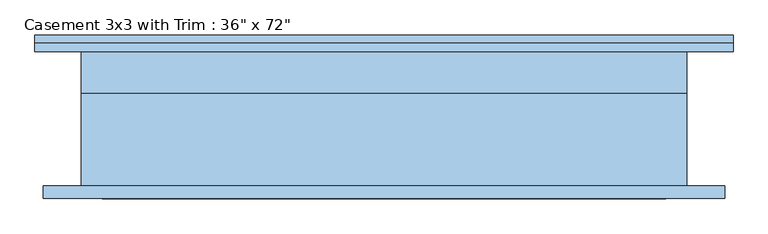
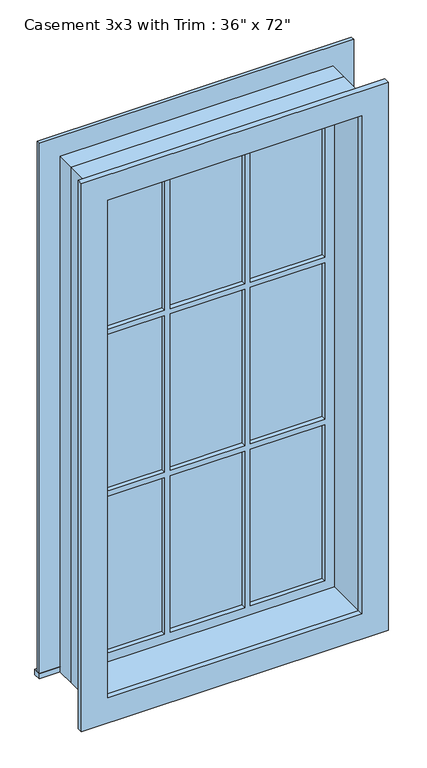
"""IFC4 building model written with IfcOpenShell, lengths in millimetres: window geometry."""

from ifc_helpers import new_model, si_unit, frame, origin, place, context, project, spatial, polyline, outline, extrude, source, transform, mapped, element, save


def window_8b323df3(model_context):
    return source(origin(), model_context, "Body", "SweptSolid", [
        extrude(outline(polyline([(-527.05, 127.0), (527.05, 127.0), (527.05, 101.6), (-527.05, 101.6), (-527.05, 127.0)])), frame((0.0, 0.0, 304.8), z_axis=(0.0, 0.0, 1.0), x_axis=(1.0, 0.0, 0.0)), (0.0, 0.0, 1.0), 19.05),
        extrude(outline(polyline([(2114.55, -438.15), (2114.55, 438.15), (323.85, 438.15), (323.85, 527.05), (2203.45, 527.05), (2203.45, -527.05), (323.85, -527.05), (323.85, -438.15), (2114.55, -438.15)])), frame((0.0, 101.6, 0.0), z_axis=(0.0, 1.0, 0.0), x_axis=(0.0, 0.0, 1.0)), (0.0, 0.0, 1.0), 12.7),
        extrude(outline(polyline([(143.9333333, 66.675), (393.7, 66.675), (393.7, 53.975), (143.9333333, 53.975), (143.9333333, 66.675)])), frame((0.0, 0.0, 1515.5333333), z_axis=(0.0, 0.0, 1.0), x_axis=(1.0, 0.0, 0.0)), (0.0, 0.0, 1.0), 554.5666667),
        extrude(outline(polyline([(-124.8833333, 66.675), (124.8833333, 66.675), (124.8833333, 53.975), (-124.8833333, 53.975), (-124.8833333, 66.675)])), frame((0.0, 0.0, 1515.5333333), z_axis=(0.0, 0.0, 1.0), x_axis=(1.0, 0.0, 0.0)), (0.0, 0.0, 1.0), 554.5666667),
        extrude(outline(polyline([(-393.7, 66.675), (-143.9333333, 66.675), (-143.9333333, 53.975), (-393.7, 53.975), (-393.7, 66.675)])), frame((0.0, 0.0, 1515.5333333), z_axis=(0.0, 0.0, 1.0), x_axis=(1.0, 0.0, 0.0)), (0.0, 0.0, 1.0), 554.5666667),
        extrude(outline(polyline([(-393.7, 66.675), (-143.9333333, 66.675), (-143.9333333, 53.975), (-393.7, 53.975), (-393.7, 66.675)])), frame((0.0, 0.0, 941.9166667), z_axis=(0.0, 0.0, 1.0), x_axis=(1.0, 0.0, 0.0)), (0.0, 0.0, 1.0), 554.5666667),
        extrude(outline(polyline([(-124.8833333, 66.675), (124.8833333, 66.675), (124.8833333, 53.975), (-124.8833333, 53.975), (-124.8833333, 66.675)])), frame((0.0, 0.0, 941.9166667), z_axis=(0.0, 0.0, 1.0), x_axis=(1.0, 0.0, 0.0)), (0.0, 0.0, 1.0), 554.5666667),
        extrude(outline(polyline([(143.9333333, 66.675), (393.7, 66.675), (393.7, 53.975), (143.9333333, 53.975), (143.9333333, 66.675)])), frame((0.0, 0.0, 941.9166667), z_axis=(0.0, 0.0, 1.0), x_axis=(1.0, 0.0, 0.0)), (0.0, 0.0, 1.0), 554.5666667),
        extrude(outline(polyline([(143.9333333, 66.675), (393.7, 66.675), (393.7, 53.975), (143.9333333, 53.975), (143.9333333, 66.675)])), frame((0.0, 0.0, 368.3), z_axis=(0.0, 0.0, 1.0), x_axis=(1.0, 0.0, 0.0)), (0.0, 0.0, 1.0), 554.5666667),
        extrude(outline(polyline([(-124.8833333, 66.675), (124.8833333, 66.675), (124.8833333, 53.975), (-124.8833333, 53.975), (-124.8833333, 66.675)])), frame((0.0, 0.0, 368.3), z_axis=(0.0, 0.0, 1.0), x_axis=(1.0, 0.0, 0.0)), (0.0, 0.0, 1.0), 554.5666667),
        extrude(outline(polyline([(-393.7, 66.675), (-143.9333333, 66.675), (-143.9333333, 53.975), (-393.7, 53.975), (-393.7, 66.675)])), frame((0.0, 0.0, 368.3), z_axis=(0.0, 0.0, 1.0), x_axis=(1.0, 0.0, 0.0)), (0.0, 0.0, 1.0), 554.5666667),
        extrude(outline(polyline([(2190.75, 514.35), (2190.75, -514.35), (247.65, -514.35), (247.65, 514.35), (2190.75, 514.35)]), holes=[polyline([(2101.85, 425.45), (336.55, 425.45), (336.55, -425.45), (2101.85, -425.45), (2101.85, 425.45)])]), frame((0.0, -120.65, 0.0), z_axis=(0.0, 1.0, 0.0), x_axis=(0.0, 0.0, 1.0)), (0.0, 0.0, 1.0), 19.05),
        extrude(outline(polyline([(2114.55, -438.15), (323.85, -438.15), (323.85, 438.15), (2114.55, 438.15), (2114.55, -438.15)]), holes=[polyline([(2070.1, -143.9333333), (1515.5333333, -143.9333333), (1515.5333333, -393.7), (2070.1, -393.7), (2070.1, -143.9333333)]), polyline([(1496.4833333, -143.9333333), (941.9166667, -143.9333333), (941.9166667, -393.7), (1496.4833333, -393.7), (1496.4833333, -143.9333333)]), polyline([(922.8666667, -143.9333333), (368.3, -143.9333333), (368.3, -393.7), (922.8666667, -393.7), (922.8666667, -143.9333333)]), polyline([(2070.1, 124.8833333), (1515.5333333, 124.8833333), (1515.5333333, -124.8833333), (2070.1, -124.8833333), (2070.1, 124.8833333)]), polyline([(1496.4833333, 124.8833333), (941.9166667, 124.8833333), (941.9166667, -124.8833333), (1496.4833333, -124.8833333), (1496.4833333, 124.8833333)]), polyline([(922.8666667, 124.8833333), (368.3, 124.8833333), (368.3, -124.8833333), (922.8666667, -124.8833333), (922.8666667, 124.8833333)]), polyline([(2070.1, 393.7), (1515.5333333, 393.7), (1515.5333333, 143.9333333), (2070.1, 143.9333333), (2070.1, 393.7)]), polyline([(1496.4833333, 393.7), (941.9166667, 393.7), (941.9166667, 143.9333333), (1496.4833333, 143.9333333), (1496.4833333, 393.7)]), polyline([(922.8666667, 393.7), (368.3, 393.7), (368.3, 143.9333333), (922.8666667, 143.9333333), (922.8666667, 393.7)])]), frame((0.0, 38.1, 0.0), z_axis=(0.0, 1.0, 0.0), x_axis=(0.0, 0.0, 1.0)), (0.0, 0.0, 1.0), 44.45),
        extrude(outline(polyline([(2133.6, -457.2), (304.8, -457.2), (304.8, 457.2), (2133.6, 457.2), (2133.6, -457.2)]), holes=[polyline([(2101.85, -425.45), (2101.85, 425.45), (336.55, 425.45), (336.55, -425.45), (2101.85, -425.45)])]), frame((0.0, -101.6, 0.0), z_axis=(0.0, 1.0, 0.0), x_axis=(0.0, 0.0, 1.0)), (0.0, 0.0, 1.0), 139.7),
        extrude(outline(polyline([(2133.6, 457.2), (2133.6, -457.2), (304.8, -457.2), (304.8, 457.2), (2133.6, 457.2)]), holes=[polyline([(2114.55, 438.15), (323.85, 438.15), (323.85, -438.15), (2114.55, -438.15), (2114.55, 438.15)])]), frame((0.0, 38.1, 0.0), z_axis=(0.0, 1.0, 0.0), x_axis=(0.0, 0.0, 1.0)), (0.0, 0.0, 1.0), 63.5),
    ])


if __name__ == "__main__":
    model = new_model("IFC4")
    model_context = context("Model", 3, world=origin())
    ifc_project = project(units=[si_unit("LENGTHUNIT", "METRE", prefix="MILLI")], contexts=[model_context])
    site = spatial("IfcSite", under=ifc_project)
    building = spatial("IfcBuilding", under=site)
    placement = place(None, origin())
    window_shape = window_8b323df3(model_context)
    element("IfcWindow", 1, ObjectType="Casement 3x3 with Trim : 36\" x 72\"", at=placement, inside=building, context=model_context, shape_type="MappedRepresentation", body=[
        mapped(window_shape, transform((0.0, 0.0, 0.0), x_axis=(1.0, 0.0, 0.0), y_axis=(0.0, 1.0, 0.0), z_axis=(0.0, 0.0, 1.0))),
    ])
    save(model, "model.ifc")

# Revit data of these elements
# Type "Casement 3x3 with Trim : 36\" x 72\""
#   Type Mark = "15"
#   Construction Type Id = "GSP4R"
#   Assembly Code = "B2020100"
#   Analytic Construction = "1/8 in Pilkington single glazing"
#   Visual Light Transmittance = 0.9
#   Solar Heat Gain Coefficient = 0.78
#   Heat Transfer Coefficient (U) = 0.6496 BTU/(h·ft²·°F)
#   Height = 6' - 0"
#   Default Sill Height = 1' - 0"
#   Trim Projection - Ext. = 0' - 0 1/2"
#   Trim Projection - Int. = 0' - 0 3/4"
#   Trim Width - Exterior = 0' - 3 1/2"
#   Trim Width - Interior = 0' - 3 1/2"
#   Width = 3' - 0"
#   Window Inset = 0' - 0 3/4"
#   Define Thermal Properties by = 1
#   Glass Pane Material = Glass
#   Sash Material = Sash
#   Trim Exterior Material = Trim
#   Trim Interior Material = Trim
#   Wall Closure = (empty or 0)
# Element 1 (IfcWindow, "Casement 3x3 with Trim : 36\" x 72\"")
#   Materials on its faces: "Sash", "Glass", "Trim"
# Materials
#   "Glass": class "Glass", colour RGB 0 128 192, transparency 0.75, Description = "Soda Lime Glass", Cost = 0
#   "Sash": class "Wood", colour RGB 224 178 126, transparency 0
#   "Trim": class "Wood", colour RGB 224 178 126, transparency 0
